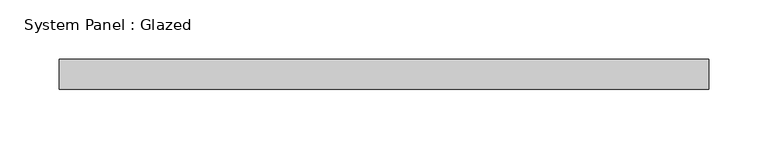
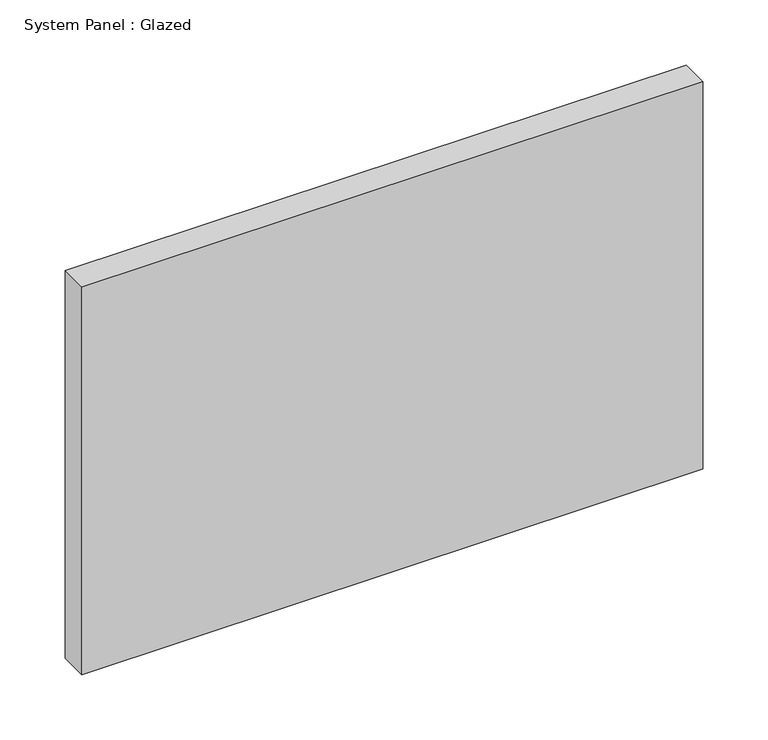
"""IFC4 building model written with IfcOpenShell, lengths in millimetres: plate geometry, System Panel : Glazed."""

from ifc_helpers import new_model, si_unit, origin, origin_with_axes, place, context, project, spatial, polyline, outline, extrude, source, transform, mapped, element, save


def system_panel_glazed_7f181415(model_context):
    return source(origin(), model_context, "Body", "SweptSolid", [
        extrude(outline(polyline([(274.1083333, 19.05), (-274.1083333, 19.05), (-274.1083333, 44.45), (274.1083333, 44.45), (274.1083333, 19.05)])), origin_with_axes(), (0.0, 0.0, 1.0), 361.95),
    ])


if __name__ == "__main__":
    model = new_model("IFC4")
    model_context = context("Model", 3, world=origin())
    ifc_project = project(units=[si_unit("LENGTHUNIT", "METRE", prefix="MILLI")], contexts=[model_context])
    site = spatial("IfcSite", under=ifc_project)
    building = spatial("IfcBuilding", under=site)
    placement = place(None, origin())
    system_panel_glazed_shape = system_panel_glazed_7f181415(model_context)
    element("IfcPlate", 1, ObjectType="System Panel : Glazed", at=placement, inside=building, context=model_context, shape_type="MappedRepresentation", body=[
        mapped(system_panel_glazed_shape, transform((0.0, 0.0, 0.0), x_axis=(1.0, 0.0, 0.0), y_axis=(0.0, 1.0, 0.0), z_axis=(0.0, 0.0, 1.0))),
    ])
    save(model, "model.ifc")

# Revit data of these elements
# Type "System Panel : Glazed"
#   Construction Type Id = "GSP4R"
#   Analytic Construction = "1/8 in Pilkington single glazing"
#   Visual Light Transmittance = 0.9
#   Solar Heat Gain Coefficient = 0.86
#   Heat Transfer Coefficient (U) = 1.18115 BTU/(h·ft²·°F)
# Element 1 (IfcPlate, "System Panel : Glazed")
#   Materials on its faces: "Glass"
# Materials
#   "Glass": class "Glass", colour RGB 0 128 192, transparency 0.75, Description = "Soda Lime Glass", Cost = 0
